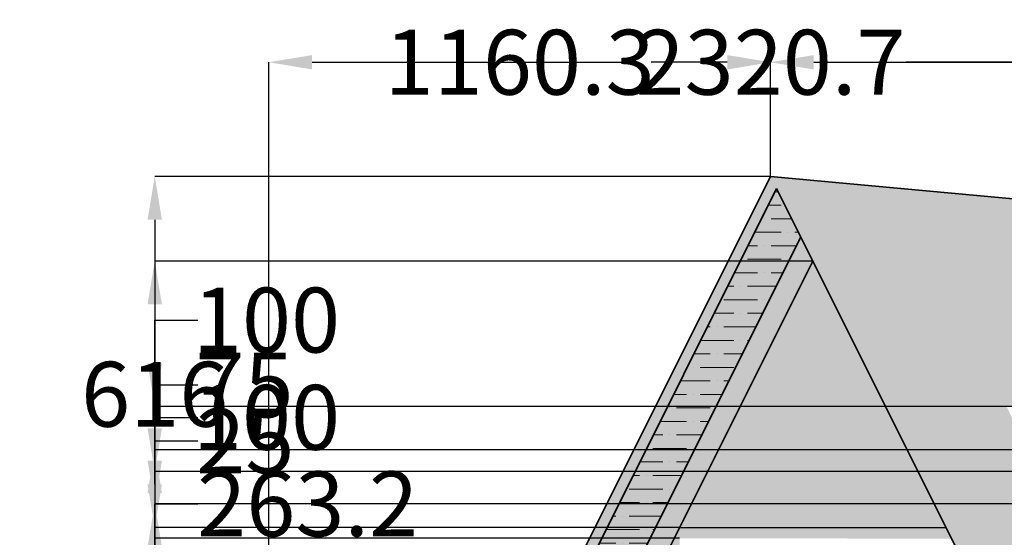
# Model space of a CAD drawing. Units: millimetres. Extents: x -504 to 6314, y 1290 to 4335.
# Tile 2 of 9: x -504 to 1774, y 3138 to 4335. Entities that reach past the tile are written whole.
import ezdxf

# ---------------------------------------------------------------- set-up
doc = ezdxf.new("R2010")
doc.units = ezdxf.units.MM
doc.header["$MEASUREMENT"] = 0
for name, color, linetype, lineweight in [('A-ANNO-DIMS', 2, 'Continuous', 18), ('A-ELEV', 7, 'Continuous', 35), ('A-ELEV-PATT', 8, 'Continuous', 13)]:
    doc.layers.add(name, color=color, linetype=linetype, lineweight=lineweight)
doc.styles.get("Standard").update_dxf_attribs({"font": 'arial.ttf'})
doc.dimstyles.get("Standard").update_dxf_attribs({"dimtxt": 150, "dimasz": 100, "dimexe": 0.18, "dimexo": 0.0625, "dimgap": 0.09, "dimtad": 0, "dimtih": 1, "dimtoh": 1, "dimdec": 0, "dimzin": 0, "dimdsep": 46, "dimtxsty": 'Standard', "dimcen": 0.09, "dimadec": 0, "dimazin": 0, "dimtfac": 1, "dimtdec": 0, "dimtofl": 0, "dimtmove": 0, "dimatfit": 3, "dimfxl": 1, "dimtolj": 1, "dimtzin": 0, "dimarcsym": 0})

# ---------------------------------------------------------------- blocks, each defined once
blk = doc.blocks.new('*D2')
at = {"layer": 'A-ANNO-DIMS', "color": 0, "lineweight": -2, "transparency": 16777216}
for p, q in [((1233.1, 3972.8), (-191.3, 3972.8)), ((-191.2, 3872.8), (-191.2, 2889.2)), ((-191.2, 1752.1), (-191.2, 2735.7)), ((72.8, 1652.1), (-191.3, 1652.1))]:
    blk.add_line(p, q, dxfattribs=at)
at = {"layer": 'A-ANNO-DIMS', "color": 0, "transparency": 16777216}
for points in [[(-207.8, 3872.8), (-174.5, 3872.8), (-191.2, 3972.8)], [(-207.8, 1752.1), (-174.5, 1752.1), (-191.2, 1652.1)]]:
    blk.add_solid(points, dxfattribs=at)
at = {"layer": 'Defpoints', "color": 0, "transparency": 16777216}
for p in [(-191.2, 3972.8), (1233.2, 3972.8), (72.8, 1652.1)]:
    blk.add_point(p, dxfattribs=at)
at = {"layer": 'A-ANNO-DIMS', "color": 0, "transparency": 16777216, "insert": (-191.2, 2812.5), "char_height": 150, "attachment_point": 5}
blk.add_mtext('\\A1;2320.7', dxfattribs=at)
blk = doc.blocks.new('*D3')
at = {"layer": 'A-ANNO-DIMS', "color": 0, "lineweight": -2, "transparency": 16777216}
for p, q in [((72.8, 1652.2), (72.8, 4237)), ((172.8, 4236.8), (348.6, 4236.8)), ((1133.2, 4236.8), (957.4, 4236.8)), ((1233.2, 3972.8), (1233.2, 4237))]:
    blk.add_line(p, q, dxfattribs=at)
at = {"layer": 'A-ANNO-DIMS', "color": 0, "transparency": 16777216}
for points in [[(172.8, 4253.4), (172.8, 4220.1), (72.8, 4236.8)], [(1133.2, 4253.4), (1133.2, 4220.1), (1233.2, 4236.8)]]:
    blk.add_solid(points, dxfattribs=at)
at = {"layer": 'Defpoints', "color": 0, "transparency": 16777216}
for p in [(1233.2, 4236.8), (1233.2, 3972.8), (72.8, 1652.1)]:
    blk.add_point(p, dxfattribs=at)
at = {"layer": 'A-ANNO-DIMS', "color": 0, "transparency": 16777216, "insert": (653, 4236.8), "char_height": 150, "attachment_point": 5}
blk.add_mtext('\\A1;1160.3', dxfattribs=at)
blk = doc.blocks.new('*D4')
at = {"layer": 'A-ANNO-DIMS', "color": 0, "lineweight": -2, "transparency": 16777216}
for p, q in [((1233.2, 3972.8), (1233.2, 4237)), ((1333.2, 4236.8), (1966.1, 4236.8)), ((3224.5, 4236.8), (2591.5, 4236.8)), ((3324.5, 3780.7), (3324.5, 4237))]:
    blk.add_line(p, q, dxfattribs=at)
at = {"layer": 'A-ANNO-DIMS', "color": 0, "transparency": 16777216}
for points in [[(1333.2, 4253.4), (1333.2, 4220.1), (1233.2, 4236.8)], [(3224.5, 4253.4), (3224.5, 4220.1), (3324.5, 4236.8)]]:
    blk.add_solid(points, dxfattribs=at)
at = {"layer": 'Defpoints', "color": 0, "transparency": 16777216}
for p in [(3324.5, 4236.8), (1233.2, 3972.8), (3324.5, 3780.6)]:
    blk.add_point(p, dxfattribs=at)
at = {"layer": 'A-ANNO-DIMS', "color": 0, "transparency": 16777216, "insert": (2278.8, 4236.8), "char_height": 150, "attachment_point": 5}
blk.add_mtext('\\A1;2091.3', dxfattribs=at)
blk = doc.blocks.new('*D6')
at = {"layer": 'A-ANNO-DIMS', "color": 0, "lineweight": -2, "transparency": 16777216}
for p, q in [((72.8, 1652.2), (72.8, 4237)), ((172.8, 4236.8), (920.4, 4236.8)), ((2293.5, 4236.8), (1545.9, 4236.8)), ((2393.5, 1652.2), (2393.5, 4237))]:
    blk.add_line(p, q, dxfattribs=at)
at = {"layer": 'A-ANNO-DIMS', "color": 0, "transparency": 16777216}
for points in [[(172.8, 4253.4), (172.8, 4220.1), (72.8, 4236.8)], [(2293.5, 4253.4), (2293.5, 4220.1), (2393.5, 4236.8)]]:
    blk.add_solid(points, dxfattribs=at)
at = {"layer": 'Defpoints', "color": 0, "transparency": 16777216}
for p in [(2393.5, 4236.8), (72.8, 1652.1), (2393.5, 1652.1)]:
    blk.add_point(p, dxfattribs=at)
at = {"layer": 'A-ANNO-DIMS', "color": 0, "transparency": 16777216, "insert": (1233.2, 4236.8), "char_height": 150, "attachment_point": 5}
blk.add_mtext('\\A1;2320.7', dxfattribs=at)
blk = doc.blocks.new('*D19')
at = {"layer": 'A-ANNO-DIMS', "color": 0, "lineweight": -2, "transparency": 16777216}
for p, q in [((-191.2, 3261.1), (-191.2, 3361.1)), ((-191.2, 3361.1), (-91.2, 3361.1)), ((1022.9, 3161.1), (-191.3, 3161.1)), ((1022.9, 3136.1), (-191.3, 3136.1)), ((-191.2, 3036.1), (-191.2, 2936.1))]:
    blk.add_line(p, q, dxfattribs=at)
at = {"layer": 'A-ANNO-DIMS', "color": 0, "transparency": 16777216}
for points in [[(-207.8, 3261.1), (-174.5, 3261.1), (-191.2, 3161.1)], [(-207.8, 3036.1), (-174.5, 3036.1), (-191.2, 3136.1)]]:
    blk.add_solid(points, dxfattribs=at)
at = {"layer": 'Defpoints', "color": 0, "transparency": 16777216}
for p in [(-191.2, 3161.1), (1023, 3161.1), (1023, 3136.1)]:
    blk.add_point(p, dxfattribs=at)
at = {"layer": 'A-ANNO-DIMS', "color": 0, "transparency": 16777216, "insert": (18.2, 3361.1), "char_height": 150, "attachment_point": 5}
blk.add_mtext('\\A1;25', dxfattribs=at)
blk = doc.blocks.new('*D20')
at = {"layer": 'A-ANNO-DIMS', "color": 0, "lineweight": -2, "transparency": 16777216}
for p, q in [((1330.9, 3777.1), (-191.3, 3777.1)), ((-191.2, 3677.1), (-191.2, 3545.8)), ((-191.2, 3261.1), (-191.2, 3392.4)), ((1022.9, 3161.1), (-191.3, 3161.1))]:
    blk.add_line(p, q, dxfattribs=at)
at = {"layer": 'A-ANNO-DIMS', "color": 0, "transparency": 16777216}
for points in [[(-207.8, 3677.1), (-174.5, 3677.1), (-191.2, 3777.1)], [(-207.8, 3261.1), (-174.5, 3261.1), (-191.2, 3161.1)]]:
    blk.add_solid(points, dxfattribs=at)
at = {"layer": 'Defpoints', "color": 0, "transparency": 16777216}
for p in [(-191.2, 3777.1), (1331, 3777.1), (1023, 3161.1)]:
    blk.add_point(p, dxfattribs=at)
at = {"layer": 'A-ANNO-DIMS', "color": 0, "transparency": 16777216, "insert": (-191.2, 3469.1), "char_height": 150, "attachment_point": 5}
blk.add_mtext('\\A1;616', dxfattribs=at)
blk = doc.blocks.new('*D28')
at = {"layer": 'A-ANNO-DIMS', "color": 0, "lineweight": -2, "transparency": 16777216}
for p, q in [((-191.2, 3540.7), (-191.2, 3640.7)), ((-191.2, 3640.7), (-91.2, 3640.7)), ((4308.5, 3440.7), (-191.3, 3440.7)), ((4304.4, 3340.7), (-191.3, 3340.7)), ((-191.2, 3240.7), (-191.2, 3140.7))]:
    blk.add_line(p, q, dxfattribs=at)
at = {"layer": 'A-ANNO-DIMS', "color": 0, "transparency": 16777216}
for points in [[(-207.8, 3540.7), (-174.5, 3540.7), (-191.2, 3440.7)], [(-207.8, 3240.7), (-174.5, 3240.7), (-191.2, 3340.7)]]:
    blk.add_solid(points, dxfattribs=at)
at = {"layer": 'Defpoints', "color": 0, "transparency": 16777216}
for p in [(-191.2, 3440.7), (4308.6, 3440.7), (4304.5, 3340.7)]:
    blk.add_point(p, dxfattribs=at)
at = {"layer": 'A-ANNO-DIMS', "color": 0, "transparency": 16777216, "insert": (67.3, 3640.7), "char_height": 150, "attachment_point": 5}
blk.add_mtext('\\A1;100', dxfattribs=at)
blk = doc.blocks.new('*D32')
at = {"layer": 'A-ANNO-DIMS', "color": 0, "lineweight": -2, "transparency": 16777216}
for p, q in [((-191.2, 3115.7), (-191.2, 3215.7)), ((-191.2, 3215.7), (-91.2, 3215.7)), ((2963.6, 3115.7), (-191.3, 3115.7)), ((-191.2, 2952.5), (-191.2, 3015.7)), ((2963.6, 2852.5), (-191.3, 2852.5))]:
    blk.add_line(p, q, dxfattribs=at)
at = {"layer": 'A-ANNO-DIMS', "color": 0, "transparency": 16777216}
for points in [[(-207.8, 3015.7), (-174.5, 3015.7), (-191.2, 3115.7)], [(-207.8, 2952.5), (-174.5, 2952.5), (-191.2, 2852.5)]]:
    blk.add_solid(points, dxfattribs=at)
at = {"layer": 'Defpoints', "color": 0, "transparency": 16777216}
for p in [(-191.2, 3115.7), (2963.6, 3115.7), (2963.6, 2852.5)]:
    blk.add_point(p, dxfattribs=at)
at = {"layer": 'A-ANNO-DIMS', "color": 0, "transparency": 16777216, "insert": (162.5, 3215.7), "char_height": 150, "attachment_point": 5}
blk.add_mtext('\\A1;263.2', dxfattribs=at)
blk = doc.blocks.new('*D33')
at = {"layer": 'A-ANNO-DIMS', "color": 0, "lineweight": -2, "transparency": 16777216}
for p, q in [((-191.2, 3315.7), (-191.2, 3415.7)), ((-191.2, 3415.7), (-91.2, 3415.7)), ((2963.6, 3215.7), (-191.3, 3215.7)), ((2963.6, 3115.7), (-191.3, 3115.7)), ((-191.2, 3015.7), (-191.2, 2915.7))]:
    blk.add_line(p, q, dxfattribs=at)
at = {"layer": 'A-ANNO-DIMS', "color": 0, "transparency": 16777216}
for points in [[(-207.8, 3315.7), (-174.5, 3315.7), (-191.2, 3215.7)], [(-207.8, 3015.7), (-174.5, 3015.7), (-191.2, 3115.7)]]:
    blk.add_solid(points, dxfattribs=at)
at = {"layer": 'Defpoints', "color": 0, "transparency": 16777216}
for p in [(-191.2, 3215.7), (2963.6, 3215.7), (2963.6, 3115.7)]:
    blk.add_point(p, dxfattribs=at)
at = {"layer": 'A-ANNO-DIMS', "color": 0, "transparency": 16777216, "insert": (67.3, 3415.7), "char_height": 150, "attachment_point": 5}
blk.add_mtext('\\A1;100', dxfattribs=at)
blk = doc.blocks.new('*D34')
at = {"layer": 'A-ANNO-DIMS', "color": 0, "lineweight": -2, "transparency": 16777216}
for p, q in [((-191.2, 3390.7), (-191.2, 3490.7)), ((-191.2, 3490.7), (-91.2, 3490.7)), ((2963.6, 3290.7), (-191.3, 3290.7)), ((2963.6, 3215.7), (-191.3, 3215.7)), ((-191.2, 3115.7), (-191.2, 3015.7))]:
    blk.add_line(p, q, dxfattribs=at)
at = {"layer": 'A-ANNO-DIMS', "color": 0, "transparency": 16777216}
for points in [[(-207.8, 3390.7), (-174.5, 3390.7), (-191.2, 3290.7)], [(-207.8, 3115.7), (-174.5, 3115.7), (-191.2, 3215.7)]]:
    blk.add_solid(points, dxfattribs=at)
at = {"layer": 'Defpoints', "color": 0, "transparency": 16777216}
for p in [(-191.2, 3290.7), (2963.6, 3290.7), (2963.6, 3215.7)]:
    blk.add_point(p, dxfattribs=at)
at = {"layer": 'A-ANNO-DIMS', "color": 0, "transparency": 16777216, "insert": (16.3, 3490.7), "char_height": 150, "attachment_point": 5}
blk.add_mtext('\\A1;75', dxfattribs=at)

msp = doc.modelspace()

# ---------------------------------------------------------------- hatches: boundary and pattern name
at = {"layer": 'A-ELEV-PATT'}
for points in [[(3324.48, 3780.626), (1233.163, 3972.781), (72.835, 1652.125), (2393.491, 1652.125), (2355.991, 1727.125), (138.286, 1727.125), (1247.138, 3944.83), (2393.491, 1652.125), (2840.705, 1652.125), (2403.888, 2525.758), (2236.182, 2525.758), (2186.182, 2625.758), (2309.166, 2625.758), (1976.702, 3290.687), (1853.718, 3290.687), (1778.718, 3440.687), (3407.797, 3440.687)], [(1303.04, 3833.026), (1247.138, 3944.83), (138.286, 1727.125), (250.089, 1727.125)], [(1330.991, 3777.125), (1303.04, 3833.026), (250.089, 1727.125), (2355.991, 1727.125), (2330.991, 1777.125), (330.991, 1777.125)], [(1977.097, 2484.912), (1688.991, 2485.278), (1688.991, 3061.125), (1663.991, 3111.125), (1663.991, 2485.31), (1022.991, 2486.124), (1022.991, 3136.125), (1651.89, 3135.326), (1639.382, 3160.342), (1022.991, 3161.125), (997.991, 3111.125), (997.991, 2486.156), (685.705, 2486.552), (673.213, 2461.568), (997.991, 2461.156), (997.991, 1777.125), (1022.991, 1777.125), (1022.991, 2461.124), (1663.991, 2460.31), (1663.991, 1777.125), (1688.991, 1777.125), (1688.991, 2460.278), (1989.605, 2459.896)]]:
    msp.add_hatch(color=256, dxfattribs=at).paths.add_polyline_path(points)
h = msp.add_hatch(dxfattribs=at)
h.set_pattern_fill('ANSI36', color=256, scale=200, angle=135, style=0)
h.paths.add_polyline_path([(3324.48, 3780.626), (1233.163, 3972.781), (72.835, 1652.125), (2393.491, 1652.125), (2355.991, 1727.125), (138.286, 1727.125), (1247.138, 3944.83), (2393.491, 1652.125), (2840.705, 1652.125), (2403.888, 2525.758), (2236.182, 2525.758), (2186.182, 2625.758), (2309.166, 2625.758), (1976.702, 3290.687), (1853.718, 3290.687), (1778.718, 3440.687), (3407.797, 3440.687)])
h = msp.add_hatch(dxfattribs=at)
h.set_pattern_fill('ANSI36', color=256, scale=250, angle=135, style=0)
h.paths.add_polyline_path([(1303.04, 3833.026), (1247.138, 3944.83), (138.286, 1727.125), (250.089, 1727.125)])
h = msp.add_hatch(color=256, dxfattribs=at)
h.set_gradient(color1=(147, 149, 152), color2=(254, 204, 102), tint=1, name='HEMISPHERICAL')
h.paths.add_polyline_path([(1639.382, 3160.342), (1330.991, 3777.125), (1022.991, 3161.125)])

# ---------------------------------------------------------------- linework, layer by layer
at = {"layer": 'A-ELEV'}
for p, q in [((1233.163, 3972.781), (72.835, 1652.125)), ((1233.163, 3972.781), (3324.48, 3780.626)), ((1247.138, 3944.83), (138.286, 1727.125)), ((1247.138, 3944.83), (2393.491, 1652.125)), ((1303.04, 3833.026), (250.089, 1727.125)), ((1330.991, 3777.125), (330.991, 1777.125)), ((1022.991, 3161.125), (1639.382, 3160.342))]:
    msp.add_line(p, q, dxfattribs=at)

# ---------------------------------------------------------------- dimensions: what is measured, and where the dimension line sits
at = {"layer": 'A-ANNO-DIMS'}
for base, p1, p2, picture, middle in [((1233.163, 4236.781), (72.835, 1652.125), (1233.163, 3972.781), '*D3', (652.999, 4236.781)), ((2393.491, 4236.781), (72.835, 1652.125), (2393.491, 1652.125), '*D6', (1233.163, 4236.781)), ((3324.48, 4236.781), (1233.163, 3972.781), (3324.48, 3780.626), '*D4', (2278.822, 4236.781))]:
    dim = msp.add_linear_dim(base=base, p1=p1, p2=p2, dimstyle='Standard', override={"dimdec": 1, "dimlfac": 1, "dimrnd": 0, "dimzin": 0, "dimdsep": 46, "dimlunit": 2}, dxfattribs=at)
    dim.commit()
    dim.dimension.update_dxf_attribs({"geometry": picture, "text_midpoint": middle})
for base, p1, p2, override, picture, middle in [((-191.165, 3972.781), (72.835, 1652.125), (1233.163, 3972.781), {"dimdec": 1, "dimlfac": 1, "dimrnd": 0, "dimzin": 0, "dimdsep": 46, "dimlunit": 2}, '*D2', (-191.165, 2812.453)), ((-191.165, 3777.125), (1022.991, 3161.125), (1330.991, 3777.125), {"dimdec": 0, "dimlfac": 1, "dimrnd": 0, "dimzin": 0, "dimdsep": 46, "dimlunit": 2}, '*D20', (-191.165, 3469.125)), ((-191.165, 3440.687), (4304.463, 3340.687), (4308.57, 3440.687), {"dimdec": 0, "dimlfac": 1, "dimrnd": 0, "dimzin": 0, "dimdsep": 46, "dimlunit": 2}, '*D28', (67.315, 3640.687)), ((-191.165, 3290.687), (2963.634, 3215.687), (2963.634, 3290.687), {"dimdec": 0, "dimlfac": 1, "dimrnd": 0, "dimzin": 0, "dimdsep": 46, "dimlunit": 2}, '*D34', (16.309, 3490.687)), ((-191.165, 3215.687), (2963.634, 3115.687), (2963.634, 3215.687), {"dimdec": 0, "dimlfac": 1, "dimrnd": 0, "dimzin": 0, "dimdsep": 46, "dimlunit": 2}, '*D33', (67.315, 3415.687)), ((-191.165, 3161.125), (1022.991, 3136.125), (1022.991, 3161.125), {"dimdec": 0, "dimlfac": 1, "dimrnd": 0, "dimzin": 0, "dimdsep": 46, "dimlunit": 2}, '*D19', (18.202, 3361.125)), ((-191.165, 3115.687), (2963.634, 2852.466), (2963.634, 3115.687), {"dimdec": 1, "dimlfac": 1, "dimrnd": 0, "dimzin": 0, "dimdsep": 46, "dimlunit": 2}, '*D32', (162.523, 3215.687))]:
    dim = msp.add_linear_dim(base=base, p1=p1, p2=p2, angle=90, dimstyle='Standard', override=override, dxfattribs=at)
    dim.commit()
    dim.dimension.update_dxf_attribs({"geometry": picture, "text_midpoint": middle})

doc.saveas('drawing.dxf')
